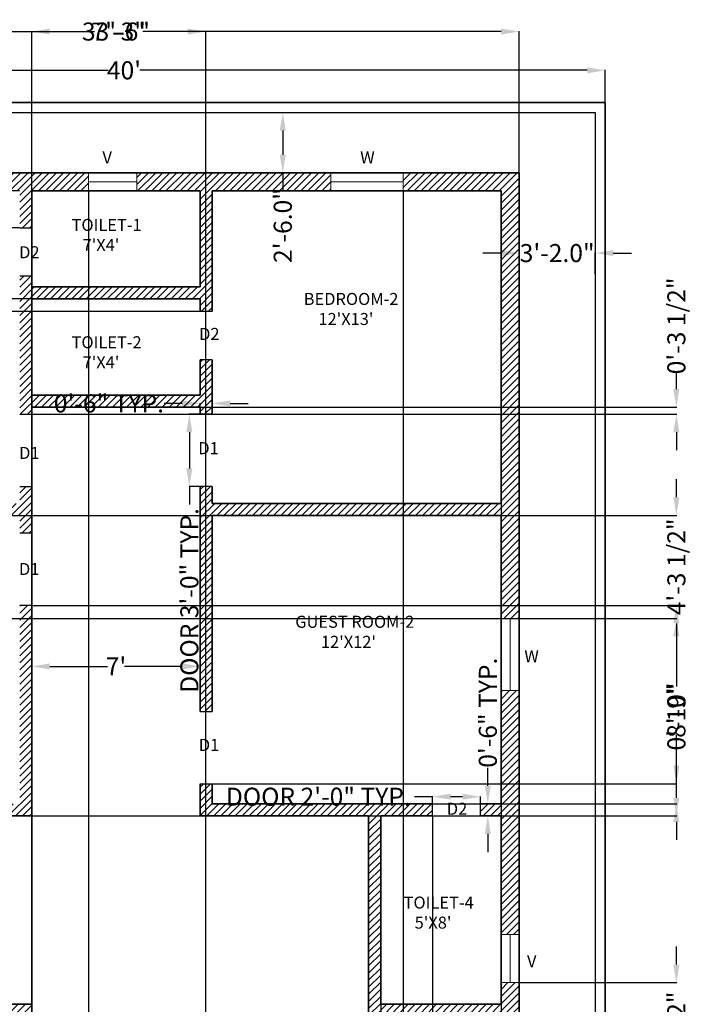
# Model space of a CAD drawing. Units: inches. Extents: x 287 to 864, y 208 to 990.
# Tile 3 of 3: x 524 to 864, y 491 to 982. Entities that reach past the tile are written whole.
import ezdxf

# ---------------------------------------------------------------- set-up
doc = ezdxf.new("R2010")
doc.units = ezdxf.units.IN
doc.header["$MEASUREMENT"] = 0
for name, color, linetype, lineweight in [('A-ANNO-DIMS', 2, 'Continuous', 18), ('A-ANNO-TEXT', 7, 'Continuous', 18), ('A-AREA-IDEN', 7, 'Continuous', 18), ('A-DOOR', 3, 'Continuous', 25), ('A-GLAZ', 4, 'Continuous', 18), ('A-SITE-WALL', 7, 'Continuous', 30), ('A-WALL', 7, 'Continuous', 35), ('C-PROP', 7, 'Continuous', 35)]:
    doc.layers.add(name, color=color, linetype=linetype, lineweight=lineweight)
doc.layers.add('A-WALL-PATT', color=240, linetype='Continuous', lineweight=13, true_color=0xed1f24)
doc.styles.get("Standard").update_dxf_attribs({"font": 'arial.ttf'})
doc.dimstyles.get("Standard").update_dxf_attribs({"dimtxt": 9, "dimasz": 9, "dimexe": 0.18, "dimexo": 0.0625, "dimgap": 0.09, "dimtad": 0, "dimdec": 1, "dimzin": 0, "dimdsep": 46, "dimlunit": 3, "dimtxsty": 'Standard', "dimcen": 0.09, "dimadec": 0, "dimazin": 0, "dimtfac": 1, "dimtdec": 1, "dimtofl": 0, "dimtmove": 0, "dimatfit": 3, "dimfxl": 1, "dimtolj": 1, "dimtzin": 0, "dimarcsym": 0})

# ---------------------------------------------------------------- blocks, each defined once
blk = doc.blocks.new('*D1')
at = {"layer": 'A-ANNO-DIMS', "color": 0, "lineweight": -2, "transparency": 16777216}
for p, q in [((335.59, 941.12), (335.59, 957.32)), ((344.59, 957.14), (567.68, 957.14)), ((806.59, 957.14), (583.5, 957.14)), ((815.59, 941.12), (815.59, 957.32))]:
    blk.add_line(p, q, dxfattribs=at)
at = {"layer": 'A-ANNO-DIMS', "color": 0, "transparency": 16777216}
for points in [[(344.59, 958.64), (344.59, 955.64), (335.59, 957.14)], [(806.59, 958.64), (806.59, 955.64), (815.59, 957.14)]]:
    blk.add_solid(points, dxfattribs=at)
at = {"layer": 'Defpoints', "color": 0, "transparency": 16777216}
for p in [(815.59, 957.14), (335.59, 941.05), (815.59, 941.05)]:
    blk.add_point(p, dxfattribs=at)
at = {"layer": 'A-ANNO-DIMS', "color": 0, "transparency": 16777216, "insert": (575.59, 957.14), "char_height": 9, "attachment_point": 5}
blk.add_mtext("\\A1;40'", dxfattribs=at)
blk = doc.blocks.new('*D4')
at = {"layer": 'A-ANNO-DIMS', "color": 0, "lineweight": -2, "transparency": 16777216}
for p, q in [((650.45, 936.05), (654.94, 936.05)), ((654.76, 927.05), (654.76, 915.05)), ((650.45, 906.05), (654.94, 906.05)), ((654.76, 906.05), (654.76, 897.05))]:
    blk.add_line(p, q, dxfattribs=at)
at = {"layer": 'A-ANNO-DIMS', "color": 0, "transparency": 16777216}
for points in [[(653.26, 927.05), (656.26, 927.05), (654.76, 936.05)], [(653.26, 915.05), (656.26, 915.05), (654.76, 906.05)]]:
    blk.add_solid(points, dxfattribs=at)
at = {"layer": 'Defpoints', "color": 0, "transparency": 16777216}
for p in [(650.39, 936.05), (650.39, 906.05), (654.76, 906.05)]:
    blk.add_point(p, dxfattribs=at)
at = {"layer": 'A-ANNO-DIMS', "color": 0, "transparency": 16777216, "insert": (654.76, 879.68), "char_height": 9, "attachment_point": 5, "rotation": 90}
blk.add_mtext('\\A1;2\'-6.0"', dxfattribs=at)
blk = doc.blocks.new('*D6')
at = {"layer": 'A-ANNO-DIMS', "color": 0, "lineweight": -2, "transparency": 16777216}
for p, q in [((529.59, 655.44), (529.59, 659.86)), ((538.59, 659.68), (567.4, 659.68)), ((604.59, 659.68), (575.78, 659.68)), ((613.59, 655.44), (613.59, 659.86))]:
    blk.add_line(p, q, dxfattribs=at)
at = {"layer": 'A-ANNO-DIMS', "color": 0, "transparency": 16777216}
for points in [[(538.59, 661.18), (538.59, 658.18), (529.59, 659.68)], [(604.59, 661.18), (604.59, 658.18), (613.59, 659.68)]]:
    blk.add_solid(points, dxfattribs=at)
at = {"layer": 'Defpoints', "color": 0, "transparency": 16777216}
for p in [(613.59, 659.68), (529.59, 655.38), (613.59, 655.38)]:
    blk.add_point(p, dxfattribs=at)
at = {"layer": 'A-ANNO-DIMS', "color": 0, "transparency": 16777216, "insert": (571.59, 659.68), "char_height": 9, "attachment_point": 5}
blk.add_mtext("\\A1;7'", dxfattribs=at)
blk = doc.blocks.new('*D7')
at = {"layer": 'A-ANNO-DIMS', "color": 0, "lineweight": -2, "transparency": 16777216}
for p, q in [((763.59, 865.94), (754.59, 865.94)), ((772.59, 855.55), (772.59, 866.12)), ((810.59, 855.55), (810.59, 866.12)), ((819.59, 865.94), (828.59, 865.94))]:
    blk.add_line(p, q, dxfattribs=at)
at = {"layer": 'A-ANNO-DIMS', "color": 0, "transparency": 16777216}
for points in [[(763.59, 867.44), (763.59, 864.44), (772.59, 865.94)], [(819.59, 867.44), (819.59, 864.44), (810.59, 865.94)]]:
    blk.add_solid(points, dxfattribs=at)
at = {"layer": 'Defpoints', "color": 0, "transparency": 16777216}
for p in [(810.59, 865.94), (772.59, 855.49), (810.59, 855.49)]:
    blk.add_point(p, dxfattribs=at)
at = {"layer": 'A-ANNO-DIMS', "color": 0, "transparency": 16777216, "insert": (791.59, 865.94), "char_height": 9, "attachment_point": 5}
blk.add_mtext('\\A1;3\'-2.0"', dxfattribs=at)
blk = doc.blocks.new('WIN-36IN')
for p, q in [((0, 9), (0, 0)), ((36, 9), (36, 0)), ((0, 4.5), (36, 4.5))]:
    blk.add_line(p, q)
blk = doc.blocks.new('VENT-24IN')
for p, q in [((0, 24), (9, 24)), ((4.5, 0), (4.5, 24)), ((0, 0), (9, 0))]:
    blk.add_line(p, q)
blk = doc.blocks.new('DOOR-OPENING-36IN')
for p, q in [((0, 36), (6, 36)), ((0, 0), (6, 0))]:
    blk.add_line(p, q)
blk = doc.blocks.new('DOOR-OPENING-24IN')
for p, q in [((0, 24), (6, 24)), ((0, 0), (6, 0))]:
    blk.add_line(p, q)
blk = doc.blocks.new('*D15')
at = {"layer": 'A-ANNO-DIMS', "color": 0, "lineweight": -2, "transparency": 16777216}
for p, q in [((613.53, 785.52), (608.01, 785.52)), ((608.19, 776.52), (608.19, 758.52)), ((613.53, 749.52), (608.01, 749.52)), ((608.19, 749.52), (608.19, 740.52))]:
    blk.add_line(p, q, dxfattribs=at)
at = {"layer": 'A-ANNO-DIMS', "color": 0, "transparency": 16777216}
for points in [[(606.69, 776.52), (609.69, 776.52), (608.19, 785.52)], [(606.69, 758.52), (609.69, 758.52), (608.19, 749.52)]]:
    blk.add_solid(points, dxfattribs=at)
at = {"layer": 'Defpoints', "color": 0, "transparency": 16777216}
for p in [(613.59, 785.52), (608.19, 749.52), (613.59, 749.52)]:
    blk.add_point(p, dxfattribs=at)
at = {"layer": 'A-ANNO-DIMS', "color": 0, "transparency": 16777216, "insert": (608.19, 692.62), "char_height": 9, "attachment_point": 5, "rotation": 90}
blk.add_mtext('\\A1;DOOR 3\'-0" TYP.', dxfattribs=at)
blk = doc.blocks.new('*D16')
at = {"layer": 'A-ANNO-DIMS', "color": 0, "lineweight": -2, "transparency": 16777216}
for p, q in [((613.59, 785.58), (613.59, 791.1)), ((619.59, 785.58), (619.59, 791.1)), ((604.59, 790.92), (595.59, 790.92)), ((628.59, 790.92), (637.59, 790.92))]:
    blk.add_line(p, q, dxfattribs=at)
at = {"layer": 'A-ANNO-DIMS', "color": 0, "transparency": 16777216}
for points in [[(604.59, 792.42), (604.59, 789.42), (613.59, 790.92)], [(628.59, 792.42), (628.59, 789.42), (619.59, 790.92)]]:
    blk.add_solid(points, dxfattribs=at)
at = {"layer": 'Defpoints', "color": 0, "transparency": 16777216}
for p in [(613.59, 790.92), (613.59, 785.52), (619.59, 785.52)]:
    blk.add_point(p, dxfattribs=at)
at = {"layer": 'A-ANNO-DIMS', "color": 0, "transparency": 16777216, "insert": (568.07, 790.92), "char_height": 9, "attachment_point": 5}
blk.add_mtext('\\A1;0\'-6" TYP.', dxfattribs=at)
blk = doc.blocks.new('*D17')
at = {"layer": 'A-ANNO-DIMS', "color": 0, "lineweight": -2, "transparency": 16777216}
for p, q in [((729.41, 594.65), (720.41, 594.65)), ((729.41, 591.12), (729.41, 594.83)), ((744.41, 594.65), (738.41, 594.65)), ((753.41, 591.12), (753.41, 594.83))]:
    blk.add_line(p, q, dxfattribs=at)
at = {"layer": 'A-ANNO-DIMS', "color": 0, "transparency": 16777216}
for points in [[(738.41, 596.15), (738.41, 593.15), (729.41, 594.65)], [(744.41, 596.15), (744.41, 593.15), (753.41, 594.65)]]:
    blk.add_solid(points, dxfattribs=at)
at = {"layer": 'Defpoints', "color": 0, "transparency": 16777216}
for p in [(729.41, 594.65), (729.41, 591.05), (753.41, 591.05)]:
    blk.add_point(p, dxfattribs=at)
at = {"layer": 'A-ANNO-DIMS', "color": 0, "transparency": 16777216, "insert": (672.51, 594.65), "char_height": 9, "attachment_point": 5}
blk.add_mtext('\\A1;DOOR 2\'-0" TYP.', dxfattribs=at)
blk = doc.blocks.new('*D18')
at = {"layer": 'A-ANNO-DIMS', "color": 0, "lineweight": -2, "transparency": 16777216}
for p, q in [((757.01, 600.05), (757.01, 609.05)), ((753.47, 591.05), (757.19, 591.05)), ((753.47, 585.05), (757.19, 585.05)), ((757.01, 576.05), (757.01, 567.05))]:
    blk.add_line(p, q, dxfattribs=at)
at = {"layer": 'A-ANNO-DIMS', "color": 0, "transparency": 16777216}
for points in [[(755.51, 600.05), (758.51, 600.05), (757.01, 591.05)], [(755.51, 576.05), (758.51, 576.05), (757.01, 585.05)]]:
    blk.add_solid(points, dxfattribs=at)
at = {"layer": 'Defpoints', "color": 0, "transparency": 16777216}
for p in [(753.41, 591.05), (757.01, 591.05), (753.41, 585.05)]:
    blk.add_point(p, dxfattribs=at)
at = {"layer": 'A-ANNO-DIMS', "color": 0, "transparency": 16777216, "insert": (757.01, 636.57), "char_height": 9, "attachment_point": 5, "rotation": 90}
blk.add_mtext('\\A1;0\'-6" TYP.', dxfattribs=at)
blk = doc.blocks.new('*D23')
at = {"layer": 'A-ANNO-DIMS', "color": 0, "lineweight": -2, "transparency": 16777216}
for p, q in [((370.59, 906.12), (370.59, 976.68)), ((379.59, 976.5), (556.04, 976.5)), ((763.59, 976.5), (587.14, 976.5)), ((772.59, 906.12), (772.59, 976.68))]:
    blk.add_line(p, q, dxfattribs=at)
at = {"layer": 'A-ANNO-DIMS', "color": 0, "transparency": 16777216}
for points in [[(379.59, 978), (379.59, 975), (370.59, 976.5)], [(763.59, 978), (763.59, 975), (772.59, 976.5)]]:
    blk.add_solid(points, dxfattribs=at)
at = {"layer": 'Defpoints', "color": 0, "transparency": 16777216}
for p in [(772.59, 976.5), (370.59, 906.05), (772.59, 906.05)]:
    blk.add_point(p, dxfattribs=at)
at = {"layer": 'A-ANNO-DIMS', "color": 0, "transparency": 16777216, "insert": (571.59, 976.5), "char_height": 9, "attachment_point": 5}
blk.add_mtext('\\A1;33\'-6"', dxfattribs=at)
blk = doc.blocks.new('*D34')
at = {"layer": 'A-ANNO-DIMS', "color": 0, "lineweight": -2, "transparency": 16777216}
for p, q in [((529.59, 896.99), (529.59, 221.42)), ((557.92, 896.99), (557.92, 221.42)), ((538.59, 221.6), (548.92, 221.6)), ((557.92, 221.6), (566.92, 221.6))]:
    blk.add_line(p, q, dxfattribs=at)
at = {"layer": 'A-ANNO-DIMS', "color": 0, "transparency": 16777216}
for points in [[(538.59, 223.1), (538.59, 220.1), (529.59, 221.6)], [(548.92, 223.1), (548.92, 220.1), (557.92, 221.6)]]:
    blk.add_solid(points, dxfattribs=at)
at = {"layer": 'Defpoints', "color": 0, "transparency": 16777216}
for p in [(529.59, 897.05), (557.92, 897.05), (557.92, 221.6)]:
    blk.add_point(p, dxfattribs=at)
at = {"layer": 'A-ANNO-DIMS', "color": 0, "transparency": 16777216, "insert": (589.53, 221.6), "char_height": 9, "attachment_point": 5}
blk.add_mtext('\\A1;2\'-4 1/2"', dxfattribs=at)
blk = doc.blocks.new('*D35')
at = {"layer": 'A-ANNO-DIMS', "color": 0, "lineweight": -2, "transparency": 16777216}
for p, q in [((714.78, 896.99), (714.78, 221.42)), ((763.59, 896.99), (763.59, 221.42)), ((723.78, 221.6), (726.95, 221.6)), ((754.59, 221.6), (751.42, 221.6))]:
    blk.add_line(p, q, dxfattribs=at)
at = {"layer": 'A-ANNO-DIMS', "color": 0, "transparency": 16777216}
for points in [[(723.78, 223.1), (723.78, 220.1), (714.78, 221.6)], [(754.59, 223.1), (754.59, 220.1), (763.59, 221.6)]]:
    blk.add_solid(points, dxfattribs=at)
at = {"layer": 'Defpoints', "color": 0, "transparency": 16777216}
for p in [(714.78, 897.05), (763.59, 897.05), (763.59, 221.6)]:
    blk.add_point(p, dxfattribs=at)
at = {"layer": 'A-ANNO-DIMS', "color": 0, "transparency": 16777216, "insert": (739.19, 221.6), "char_height": 9, "attachment_point": 5}
blk.add_mtext('\\A1;4\'-1"', dxfattribs=at)
blk = doc.blocks.new('*D36')
at = {"layer": 'A-ANNO-DIMS', "color": 0, "lineweight": -2, "transparency": 16777216}
for p, q in [((851.039945, 744.054509), (851.039945, 753.054509)), ((379.652445, 735.054509), (851.219945, 735.054509)), ((379.652445, 683.646477), (851.219945, 683.646477)), ((851.039945, 674.646477), (851.039945, 665.646477))]:
    blk.add_line(p, q, dxfattribs=at)
at = {"layer": 'A-ANNO-DIMS', "color": 0, "transparency": 16777216}
for points in [[(849.539945, 744.054509), (852.539945, 744.054509), (851.039945, 735.054509)], [(849.539945, 674.646477), (852.539945, 674.646477), (851.039945, 683.646477)]]:
    blk.add_solid(points, dxfattribs=at)
at = {"layer": 'Defpoints', "color": 0, "transparency": 16777216}
for p in [(379.589945, 735.054509), (379.589945, 683.646477), (851.039945, 683.646477)]:
    blk.add_point(p, dxfattribs=at)
at = {"layer": 'A-ANNO-DIMS', "color": 0, "transparency": 16777216, "insert": (851.039945, 709.350493), "char_height": 9, "attachment_point": 5, "rotation": 90}
blk.add_mtext('\\A1;4\'-3 1/2"', dxfattribs=at)
blk = doc.blocks.new('*D37')
at = {"layer": 'A-ANNO-DIMS', "color": 0, "lineweight": -2, "transparency": 16777216}
for p, q in [((851.04, 510.9), (851.04, 519.9)), ((772.65, 501.9), (851.22, 501.9)), ((772.65, 444.61), (851.22, 444.61)), ((851.04, 435.61), (851.04, 426.61))]:
    blk.add_line(p, q, dxfattribs=at)
at = {"layer": 'A-ANNO-DIMS', "color": 0, "transparency": 16777216}
for points in [[(849.54, 510.9), (852.54, 510.9), (851.04, 501.9)], [(849.54, 435.61), (852.54, 435.61), (851.04, 444.61)]]:
    blk.add_solid(points, dxfattribs=at)
at = {"layer": 'Defpoints', "color": 0, "transparency": 16777216}
for p in [(772.59, 501.9), (851.04, 501.9), (772.59, 444.61)]:
    blk.add_point(p, dxfattribs=at)
at = {"layer": 'A-ANNO-DIMS', "color": 0, "transparency": 16777216, "insert": (851.04, 473.26), "char_height": 9, "attachment_point": 5, "rotation": 90}
blk.add_mtext('\\A1;4\'-9 1/2"', dxfattribs=at)
blk = doc.blocks.new('*D40')
at = {"layer": 'A-ANNO-DIMS', "color": 0, "lineweight": -2, "transparency": 16777216}
for p, q in [((529.59, 360.12), (529.59, 976.68)), ((538.59, 976.5), (560.96, 976.5)), ((607.36, 976.5), (584.99, 976.5)), ((616.36, 360.12), (616.36, 976.68))]:
    blk.add_line(p, q, dxfattribs=at)
at = {"layer": 'A-ANNO-DIMS', "color": 0, "transparency": 16777216}
for points in [[(538.59, 978), (538.59, 975), (529.59, 976.5)], [(607.36, 978), (607.36, 975), (616.36, 976.5)]]:
    blk.add_solid(points, dxfattribs=at)
at = {"layer": 'Defpoints', "color": 0, "transparency": 16777216}
for p in [(616.36, 976.5), (529.59, 360.05), (616.36, 360.05)]:
    blk.add_point(p, dxfattribs=at)
at = {"layer": 'A-ANNO-DIMS', "color": 0, "transparency": 16777216, "insert": (572.97, 976.5), "char_height": 9, "attachment_point": 5}
blk.add_mtext('\\A1;7\'-3"', dxfattribs=at)
blk = doc.blocks.new('*D41')
at = {"layer": 'A-ANNO-DIMS', "color": 0, "lineweight": -2, "transparency": 16777216}
for p, q in [((851.04, 798.05), (851.04, 807.05)), ((529.65, 789.05), (851.22, 789.05)), ((529.65, 785.52), (851.22, 785.52)), ((851.04, 776.52), (851.04, 767.52))]:
    blk.add_line(p, q, dxfattribs=at)
at = {"layer": 'A-ANNO-DIMS', "color": 0, "transparency": 16777216}
for points in [[(849.54, 798.05), (852.54, 798.05), (851.04, 789.05)], [(849.54, 776.52), (852.54, 776.52), (851.04, 785.52)]]:
    blk.add_solid(points, dxfattribs=at)
at = {"layer": 'Defpoints', "color": 0, "transparency": 16777216}
for p in [(529.59, 789.05), (851.04, 789.05), (529.59, 785.52)]:
    blk.add_point(p, dxfattribs=at)
at = {"layer": 'A-ANNO-DIMS', "color": 0, "transparency": 16777216, "insert": (851.04, 829.59), "char_height": 9, "attachment_point": 5, "rotation": 90}
blk.add_mtext('\\A1;0\'-3 1/2"', dxfattribs=at)
blk = doc.blocks.new('*D42')
at = {"layer": 'A-ANNO-DIMS', "color": 0, "lineweight": -2, "transparency": 16777216}
for p, q in [((523.53, 897.05), (299.96, 897.05)), ((300.14, 888.05), (300.14, 887.59)), ((523.53, 878.59), (299.96, 878.59)), ((300.14, 878.59), (300.14, 869.59))]:
    blk.add_line(p, q, dxfattribs=at)
at = {"layer": 'A-ANNO-DIMS', "color": 0, "transparency": 16777216}
for points in [[(298.64, 888.05), (301.64, 888.05), (300.14, 897.05)], [(298.64, 887.59), (301.64, 887.59), (300.14, 878.59)]]:
    blk.add_solid(points, dxfattribs=at)
at = {"layer": 'Defpoints', "color": 0, "transparency": 16777216}
for p in [(523.59, 897.05), (300.14, 878.59), (523.59, 878.59)]:
    blk.add_point(p, dxfattribs=at)
at = {"layer": 'A-ANNO-DIMS', "color": 0, "transparency": 16777216, "insert": (300.14, 847.47), "char_height": 9, "attachment_point": 5, "rotation": 90}
blk.add_mtext('\\A1;1\'-6 1/2"', dxfattribs=at)
blk = doc.blocks.new('*D43')
at = {"layer": 'A-ANNO-DIMS', "color": 0, "lineweight": -2, "transparency": 16777216}
for p, q in [((300.14, 852.05), (300.14, 861.05)), ((613.53, 843.05), (299.96, 843.05)), ((613.53, 836.74), (299.96, 836.74)), ((300.14, 827.74), (300.14, 818.74))]:
    blk.add_line(p, q, dxfattribs=at)
at = {"layer": 'A-ANNO-DIMS', "color": 0, "transparency": 16777216}
for points in [[(298.64, 852.05), (301.64, 852.05), (300.14, 843.05)], [(298.64, 827.74), (301.64, 827.74), (300.14, 836.74)]]:
    blk.add_solid(points, dxfattribs=at)
at = {"layer": 'Defpoints', "color": 0, "transparency": 16777216}
for p in [(613.59, 843.05), (300.14, 836.74), (613.59, 836.74)]:
    blk.add_point(p, dxfattribs=at)
at = {"layer": 'A-ANNO-DIMS', "color": 0, "transparency": 16777216, "insert": (300.14, 796.2), "char_height": 9, "attachment_point": 5, "rotation": 90}
blk.add_mtext('\\A1;0\'-6 1/2"', dxfattribs=at)
blk = doc.blocks.new('*D44')
at = {"layer": 'A-ANNO-DIMS', "color": 0, "lineweight": -2, "transparency": 16777216}
for p, q in [((529.65, 690.13), (851.22, 690.13)), ((851.04, 681.13), (851.04, 649.65)), ((851.04, 594.05), (851.04, 625.54)), ((529.65, 585.05), (851.22, 585.05))]:
    blk.add_line(p, q, dxfattribs=at)
at = {"layer": 'A-ANNO-DIMS', "color": 0, "transparency": 16777216}
for points in [[(849.54, 681.13), (852.54, 681.13), (851.04, 690.13)], [(849.54, 594.05), (852.54, 594.05), (851.04, 585.05)]]:
    blk.add_solid(points, dxfattribs=at)
at = {"layer": 'Defpoints', "color": 0, "transparency": 16777216}
for p in [(529.59, 690.13), (851.04, 690.13), (529.59, 585.05)]:
    blk.add_point(p, dxfattribs=at)
at = {"layer": 'A-ANNO-DIMS', "color": 0, "transparency": 16777216, "insert": (851.04, 637.59), "char_height": 9, "attachment_point": 5, "rotation": 90}
blk.add_mtext('\\A1;8\'-9"', dxfattribs=at)
blk = doc.blocks.new('*D45')
at = {"layer": 'A-ANNO-DIMS', "color": 0, "lineweight": -2, "transparency": 16777216}
for p, q in [((851.04, 610.13), (851.04, 619.13)), ((619.65, 601.13), (851.22, 601.13)), ((619.65, 591.05), (851.22, 591.05)), ((851.04, 582.05), (851.04, 573.05))]:
    blk.add_line(p, q, dxfattribs=at)
at = {"layer": 'A-ANNO-DIMS', "color": 0, "transparency": 16777216}
for points in [[(849.54, 610.13), (852.54, 610.13), (851.04, 601.13)], [(849.54, 582.05), (852.54, 582.05), (851.04, 591.05)]]:
    blk.add_solid(points, dxfattribs=at)
at = {"layer": 'Defpoints', "color": 0, "transparency": 16777216}
for p in [(619.59, 601.13), (851.04, 601.13), (619.59, 591.05)]:
    blk.add_point(p, dxfattribs=at)
at = {"layer": 'A-ANNO-DIMS', "color": 0, "transparency": 16777216, "insert": (851.04, 634.68), "char_height": 9, "attachment_point": 5, "rotation": 90}
blk.add_mtext('\\A1;0\'-10"', dxfattribs=at)
blk = doc.blocks.new('*D47')
at = {"layer": 'A-ANNO-DIMS', "color": 0, "lineweight": -2, "transparency": 16777216}
for p, q in [((703.59, 584.99), (703.59, 221.42)), ((729.41, 584.99), (729.41, 221.42)), ((694.59, 221.6), (685.59, 221.6)), ((738.41, 221.6), (747.41, 221.6))]:
    blk.add_line(p, q, dxfattribs=at)
at = {"layer": 'A-ANNO-DIMS', "color": 0, "transparency": 16777216}
for points in [[(694.59, 223.1), (694.59, 220.1), (703.59, 221.6)], [(738.41, 223.1), (738.41, 220.1), (729.41, 221.6)]]:
    blk.add_solid(points, dxfattribs=at)
at = {"layer": 'Defpoints', "color": 0, "transparency": 16777216}
for p in [(703.59, 585.05), (729.41, 585.05), (729.41, 221.6)]:
    blk.add_point(p, dxfattribs=at)
at = {"layer": 'A-ANNO-DIMS', "color": 0, "transparency": 16777216, "insert": (716.5, 221.6), "char_height": 9, "attachment_point": 5}
blk.add_mtext('\\A1;2\'-2"', dxfattribs=at)

msp = doc.modelspace()

# ---------------------------------------------------------------- hatches: boundary and pattern name
at = {"layer": 'A-WALL-PATT'}
h = msp.add_hatch(dxfattribs=at)
h.set_pattern_fill('ANSI31', color=256, scale=20)
h.paths.add_polyline_path([(443.82, 491.05), (433.59, 491.05), (433.59, 585.05), (529.59, 585.05), (529.59, 690.13), (523.59, 690.13), (523.59, 591.05), (420.92, 591.05), (420.92, 585.05), (427.59, 585.05), (427.59, 491.05), (379.59, 491.05), (379.59, 501.9), (370.59, 501.9), (370.59, 351.05), (433.14, 351.05), (433.14, 360.05), (379.59, 360.05), (379.59, 485.05), (443.82, 485.05)])
h.paths.add_polyline_path([(616.36, 360.05), (469.14, 360.05), (469.14, 351.05), (616.36, 351.05)])
h.paths.add_polyline_path([(772.59, 647.65), (763.59, 647.65), (763.59, 591.05), (753.41, 591.05), (753.41, 585.05), (763.59, 585.05), (763.59, 525.9), (772.59, 525.9)])
h.paths.add_polyline_path([(772.59, 906.05), (714.78, 906.05), (714.78, 897.05), (763.59, 897.05), (763.59, 741.05), (619.59, 741.05), (619.59, 749.52), (613.59, 749.52), (613.59, 637.13), (619.59, 637.13), (619.59, 735.05), (763.59, 735.05), (763.59, 683.65), (772.59, 683.65)])
h.paths.add_polyline_path([(678.78, 906.05), (581.92, 906.05), (581.92, 897.05), (613.59, 897.05), (613.59, 849.05), (529.59, 849.05), (529.59, 854.59), (523.59, 854.59), (523.59, 785.52), (529.59, 785.52), (529.59, 789.05), (613.59, 789.05), (613.59, 785.52), (619.59, 785.52), (619.59, 812.74), (613.59, 812.74), (613.59, 795.05), (529.59, 795.05), (529.59, 843.05), (613.59, 843.05), (613.59, 836.74), (619.59, 836.74), (619.59, 897.05), (678.78, 897.05)])
h.paths.add_polyline_path([(557.92, 906.05), (472.99, 906.05), (472.99, 897.05), (523.59, 897.05), (523.59, 878.59), (529.59, 878.59), (529.59, 897.05), (557.92, 897.05)])
h.paths.add_polyline_path([(436.99, 906.05), (370.59, 906.05), (370.59, 683.65), (379.59, 683.65), (379.59, 735.05), (523.59, 735.05), (523.59, 726.13), (529.59, 726.13), (529.59, 749.52), (523.59, 749.52), (523.59, 741.05), (379.59, 741.05), (379.59, 897.05), (436.99, 897.05)])
h.paths.add_polyline_path([(379.59, 647.65), (370.59, 647.65), (370.59, 525.9), (379.59, 525.9), (379.59, 585.05), (396.92, 585.05), (396.92, 591.05), (379.59, 591.05)], flags=17)
h.paths.add_polyline_path([(529.59, 491.05), (515.82, 491.05), (515.82, 485.05), (523.59, 485.05), (523.59, 360.05), (529.59, 360.05)], flags=17)
h.paths.add_polyline_path([(763.59, 444.61), (772.59, 444.61), (772.59, 501.9), (763.59, 501.9), (763.59, 491.05), (703.59, 491.05), (703.59, 585.05), (729.41, 585.05), (729.41, 591.05), (619.59, 591.05), (619.59, 601.13), (613.59, 601.13), (613.59, 585.05), (697.59, 585.05), (697.59, 485.05), (763.59, 485.05)])
h.paths.add_polyline_path([(772.59, 408.61), (763.59, 408.61), (763.59, 360.05), (712.36, 360.05), (712.36, 351.05), (772.59, 351.05)])

# ---------------------------------------------------------------- linework, layer by layer
at = {"layer": 'A-SITE-WALL'}
for p, q in [((340.59, 936.05), (810.59, 936.05)), ((810.59, 936.05), (810.59, 353.19))]:
    msp.add_line(p, q, dxfattribs=at)
at = {"layer": 'A-WALL'}
for p, q in [((370.59, 906.05), (772.59, 906.05)), ((772.59, 906.05), (772.59, 351.05)), ((529.59, 897.05), (613.59, 897.05)), ((529.59, 878.59), (529.59, 897.05)), ((613.59, 897.05), (613.59, 849.05)), ((619.59, 897.05), (619.59, 836.74)), ((619.59, 897.05), (763.59, 897.05)), ((763.59, 897.05), (763.59, 741.05)), ((529.59, 849.05), (529.59, 854.59)), ((529.59, 849.05), (613.59, 849.05)), ((529.59, 843.05), (613.59, 843.05)), ((529.59, 795.05), (529.59, 843.05)), ((613.59, 843.05), (613.59, 836.74)), ((613.59, 812.74), (613.59, 795.05)), ((619.59, 812.74), (619.59, 785.52)), ((529.59, 795.05), (613.59, 795.05)), ((529.59, 789.05), (613.59, 789.05)), ((529.59, 785.52), (529.59, 789.05)), ((613.59, 789.05), (613.59, 785.52)), ((529.59, 726.13), (529.59, 749.52)), ((613.59, 749.52), (613.59, 637.13)), ((619.59, 749.52), (619.59, 741.05)), ((619.59, 741.05), (763.59, 741.05)), ((619.59, 735.05), (763.59, 735.05)), ((619.59, 735.05), (619.59, 637.13)), ((763.59, 735.05), (763.59, 591.05)), ((529.59, 585.05), (529.59, 690.13)), ((613.59, 601.13), (613.59, 585.05)), ((619.59, 601.13), (619.59, 591.05)), ((619.59, 591.05), (729.41, 591.05)), ((753.41, 591.05), (763.59, 591.05)), ((433.59, 585.05), (529.59, 585.05)), ((613.59, 585.05), (697.59, 585.05)), ((697.59, 585.05), (697.59, 485.05)), ((703.59, 585.05), (703.59, 491.05)), ((703.59, 585.05), (729.41, 585.05)), ((753.41, 585.05), (763.59, 585.05)), ((763.59, 585.05), (763.59, 491.05)), ((529.59, 491.05), (515.82, 491.05)), ((763.59, 491.05), (703.59, 491.05))]:
    msp.add_line(p, q, dxfattribs=at)
at = {"layer": 'C-PROP'}
for p, q in [((335.59, 941.05), (815.59, 941.05)), ((815.59, 941.05), (815.59, 257.05))]:
    msp.add_line(p, q, dxfattribs=at)

# ---------------------------------------------------------------- block references
at = {"layer": 'A-DOOR'}
for name, p in [('DOOR-OPENING-24IN', (523.59, 854.59)), ('DOOR-OPENING-36IN', (523.59, 749.52)), ('DOOR-OPENING-36IN', (613.59, 601.13))]:
    msp.add_blockref(name, p, dxfattribs=at)
for name, p, rotation in [('DOOR-OPENING-24IN', (619.59, 836.74), 180), ('DOOR-OPENING-36IN', (619.59, 785.52), 180), ('DOOR-OPENING-36IN', (529.59, 726.13), 180), ('DOOR-OPENING-24IN', (753.41, 585.05), 89.99999999999822)]:
    msp.add_blockref(name, p, dxfattribs=dict(at, rotation=rotation))
at = {"layer": 'A-GLAZ'}
for name, p, rotation in [('VENT-24IN', (581.92, 897.05), 89.9999999999995), ('WIN-36IN', (714.78, 906.05), 180), ('WIN-36IN', (763.59, 683.65), 269.9999999999997), ('VENT-24IN', (772.59, 525.9), 180)]:
    msp.add_blockref(name, p, dxfattribs=dict(at, rotation=rotation))

# ---------------------------------------------------------------- texts
at = {"layer": 'A-ANNO-TEXT', "char_height": 6, "attachment_point": 1}
for s, insert in [('V', (564.86, 916.65)), ('W', (693.39, 916.65)), ('D2', (523.31, 869.35)), ('D2', (613.06, 828.59)), ('D1', (612.66, 771.59)), ('D1', (523.31, 769.22)), ('D1', (523.22, 711.28)), ('W', (775.24, 667.78)), ('D1', (612.91, 623.5)), ('D2', (736.57, 591.64)), ('V', (776.56, 515.57))]:
    msp.add_mtext_dynamic_manual_height_columns(s, width=80.3005, gutter_width=1, heights=[0], dxfattribs=dict(at, insert=insert))
at = {"layer": 'A-AREA-IDEN', "char_height": 6, "attachment_point": 1}
for s, insert in [("TOILET-1\\P   7'X4'", (549.46, 882.99)), ("BEDROOM-2\\P    12'X13'", (665.22, 846.05)), ("TOILET-2\\P   7'X4'", (549.46, 824.44)), ("GUEST ROOM-2\\P       12'X12'", (660.99, 684.94)), ("TOILET-4\\P   5'X8'", (715.04, 544.82))]:
    msp.add_mtext_dynamic_manual_height_columns(s, width=80.3005, gutter_width=1, heights=[0], dxfattribs=dict(at, insert=insert))

# ---------------------------------------------------------------- dimensions: what is measured, and where the dimension line sits
at = {"layer": 'A-ANNO-DIMS'}
for base, p1, p2, override, picture, middle in [((772.59, 976.5), (370.59, 906.05), (772.59, 906.05), {"dimdec": 1, "dimlfac": 1, "dimrnd": 0, "dimzin": 1, "dimdsep": 46, "dimlunit": 4, "dimfrac": 2}, '*D23', (571.59, 976.5)), ((616.36, 976.5), (529.59, 360.05), (616.36, 360.05), {"dimdec": 1, "dimlfac": 1, "dimrnd": 0, "dimzin": 1, "dimdsep": 46, "dimlunit": 4, "dimfrac": 2}, '*D40', (572.97, 976.5)), ((815.59, 957.14), (335.59, 941.05), (815.59, 941.05), {"dimclrd": 0, "dimclre": 0, "dimclrt": 0}, '*D1', (575.59, 957.14)), ((557.92, 221.6), (529.59, 897.05), (557.92, 897.05), {"dimdec": 1, "dimlfac": 1, "dimrnd": 0, "dimzin": 1, "dimdsep": 46, "dimlunit": 4, "dimfrac": 2}, '*D34', (589.53, 221.6)), ((763.59, 221.6), (714.78, 897.05), (763.59, 897.05), {"dimdec": 1, "dimlfac": 1, "dimrnd": 0, "dimzin": 1, "dimdsep": 46, "dimlunit": 4, "dimfrac": 2}, '*D35', (739.19, 221.6)), ((810.59, 865.94), (772.59, 855.49), (810.59, 855.49), {"dimclrd": 0, "dimclre": 0, "dimclrt": 0}, '*D7', (791.59, 865.94)), ((613.59, 659.68), (529.59, 655.38), (613.59, 655.38), {"dimclrd": 0, "dimclre": 0, "dimclrt": 0}, '*D6', (571.59, 659.68)), ((729.41, 221.6), (703.59, 585.05), (729.41, 585.05), {"dimdec": 1, "dimlfac": 1, "dimrnd": 0, "dimzin": 1, "dimdsep": 46, "dimlunit": 4, "dimfrac": 2}, '*D47', (716.5, 221.6))]:
    dim = msp.add_linear_dim(base=base, p1=p1, p2=p2, dimstyle='Standard', override=override, dxfattribs=at)
    dim.commit()
    dim.dimension.update_dxf_attribs({"geometry": picture, "text_midpoint": middle})
for base, p1, p2, override, picture, middle in [((654.76, 906.05), (650.39, 936.05), (650.39, 906.05), {"dimclrd": 0, "dimclre": 0, "dimclrt": 0}, '*D4', (654.76, 879.68)), ((300.14, 878.59), (523.59, 897.05), (523.59, 878.59), {"dimdec": 1, "dimlfac": 1, "dimrnd": 0, "dimzin": 1, "dimdsep": 46, "dimlunit": 4, "dimfrac": 2}, '*D42', (300.14, 847.47)), ((300.14, 836.74), (613.59, 843.05), (613.59, 836.74), {"dimdec": 1, "dimlfac": 1, "dimrnd": 0, "dimzin": 1, "dimdsep": 46, "dimlunit": 4, "dimfrac": 2}, '*D43', (300.14, 796.2)), ((851.04, 789.05), (529.59, 785.52), (529.59, 789.05), {"dimdec": 1, "dimlfac": 1, "dimrnd": 0, "dimzin": 1, "dimdsep": 46, "dimlunit": 4, "dimfrac": 2}, '*D41', (851.04, 829.59)), ((851.04, 683.65), (379.59, 735.05), (379.59, 683.65), {"dimdec": 1, "dimlfac": 1, "dimrnd": 0, "dimzin": 1, "dimdsep": 46, "dimlunit": 4, "dimfrac": 2}, '*D36', (851.04, 709.35)), ((851.04, 690.13), (529.59, 585.05), (529.59, 690.13), {"dimdec": 1, "dimlfac": 1, "dimrnd": 0, "dimzin": 1, "dimdsep": 46, "dimlunit": 4, "dimfrac": 2}, '*D44', (851.04, 637.59)), ((851.04, 601.13), (619.59, 591.05), (619.59, 601.13), {"dimdec": 1, "dimlfac": 1, "dimrnd": 0, "dimzin": 1, "dimdsep": 46, "dimlunit": 4, "dimfrac": 2}, '*D45', (851.04, 634.68)), ((851.04, 501.9), (772.59, 444.61), (772.59, 501.9), {"dimdec": 1, "dimlfac": 1, "dimrnd": 0, "dimzin": 1, "dimdsep": 46, "dimlunit": 4, "dimfrac": 2}, '*D37', (851.04, 473.26))]:
    dim = msp.add_linear_dim(base=base, p1=p1, p2=p2, angle=90, dimstyle='Standard', override=override, dxfattribs=at)
    dim.commit()
    dim.dimension.update_dxf_attribs({"geometry": picture, "text_midpoint": middle})
for base, p1, p2, angle, text, picture, middle in [((613.59, 790.92), (619.59, 785.52), (613.59, 785.52), 180, '<> TYP.', '*D16', (568.07, 790.92)), ((608.19, 749.52), (613.59, 785.52), (613.59, 749.52), 270, 'DOOR <> TYP.', '*D15', (608.19, 692.62)), ((757.01, 591.05), (753.41, 585.05), (753.41, 591.05), 90, '<> TYP.', '*D18', (757.01, 636.57)), ((729.41, 594.65), (753.41, 591.05), (729.41, 591.05), 180, 'DOOR <> TYP.', '*D17', (672.51, 594.65))]:
    dim = msp.add_linear_dim(base=base, p1=p1, p2=p2, angle=angle, text=text, dimstyle='Standard', override={"dimdec": 1, "dimlfac": 1, "dimrnd": 0, "dimzin": 1, "dimdsep": 46, "dimlunit": 4, "dimfrac": 2}, dxfattribs=at)
    dim.commit()
    dim.dimension.update_dxf_attribs({"geometry": picture, "text_midpoint": middle})

doc.saveas('drawing.dxf')
